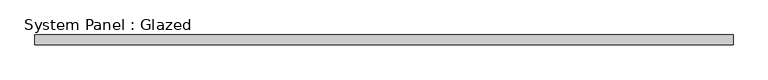
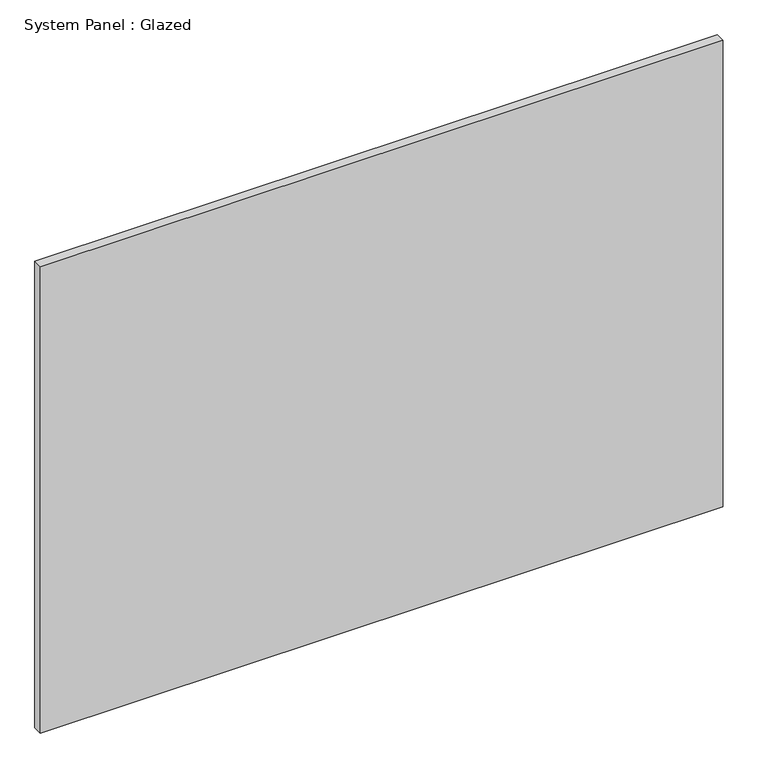
"""IFC4 building model written with IfcOpenShell, lengths in millimetres: plate geometry, System Panel : Glazed."""

from ifc_helpers import new_model, si_unit, origin, origin_with_axes, place, context, project, spatial, polyline, outline, extrude, source, transform, mapped, element, save


def system_panel_glazed_7c3c2ece(model_context):
    return source(origin(), model_context, "Body", "SweptSolid", [
        extrude(outline(polyline([(914.4, 19.05), (-914.4, 19.05), (-914.4, 44.45), (914.4, 44.45), (914.4, 19.05)])), origin_with_axes(), (0.0, 0.0, 1.0), 1320.8),
    ])


if __name__ == "__main__":
    model = new_model("IFC4")
    model_context = context("Model", 3, world=origin())
    ifc_project = project(units=[si_unit("LENGTHUNIT", "METRE", prefix="MILLI")], contexts=[model_context])
    site = spatial("IfcSite", under=ifc_project)
    building = spatial("IfcBuilding", under=site)
    placement = place(None, origin())
    system_panel_glazed_shape = system_panel_glazed_7c3c2ece(model_context)
    element("IfcPlate", 1, ObjectType="System Panel : Glazed", at=placement, inside=building, context=model_context, shape_type="MappedRepresentation", body=[
        mapped(system_panel_glazed_shape, transform((0.0, 0.0, 0.0), x_axis=(1.0, 0.0, 0.0), y_axis=(0.0, 1.0, 0.0), z_axis=(0.0, 0.0, 1.0))),
    ])
    save(model, "model.ifc")

# Revit data of these elements
# Type "System Panel : Glazed"
#   Construction Type Id = "GSP4R"
#   Analytic Construction = "1/8 in Pilkington single glazing"
#   Visual Light Transmittance = 0.9
#   Solar Heat Gain Coefficient = 0.86
#   Heat Transfer Coefficient (U) = 1.18115 BTU/(h·ft²·°F)
# Element 1 (IfcPlate, "System Panel : Glazed")
#   Materials on its faces: "Glass"
# Materials
#   "Glass": class "Glass", colour RGB 0 128 192, transparency 0.75, Description = "Soda Lime Glass", Cost = 0
